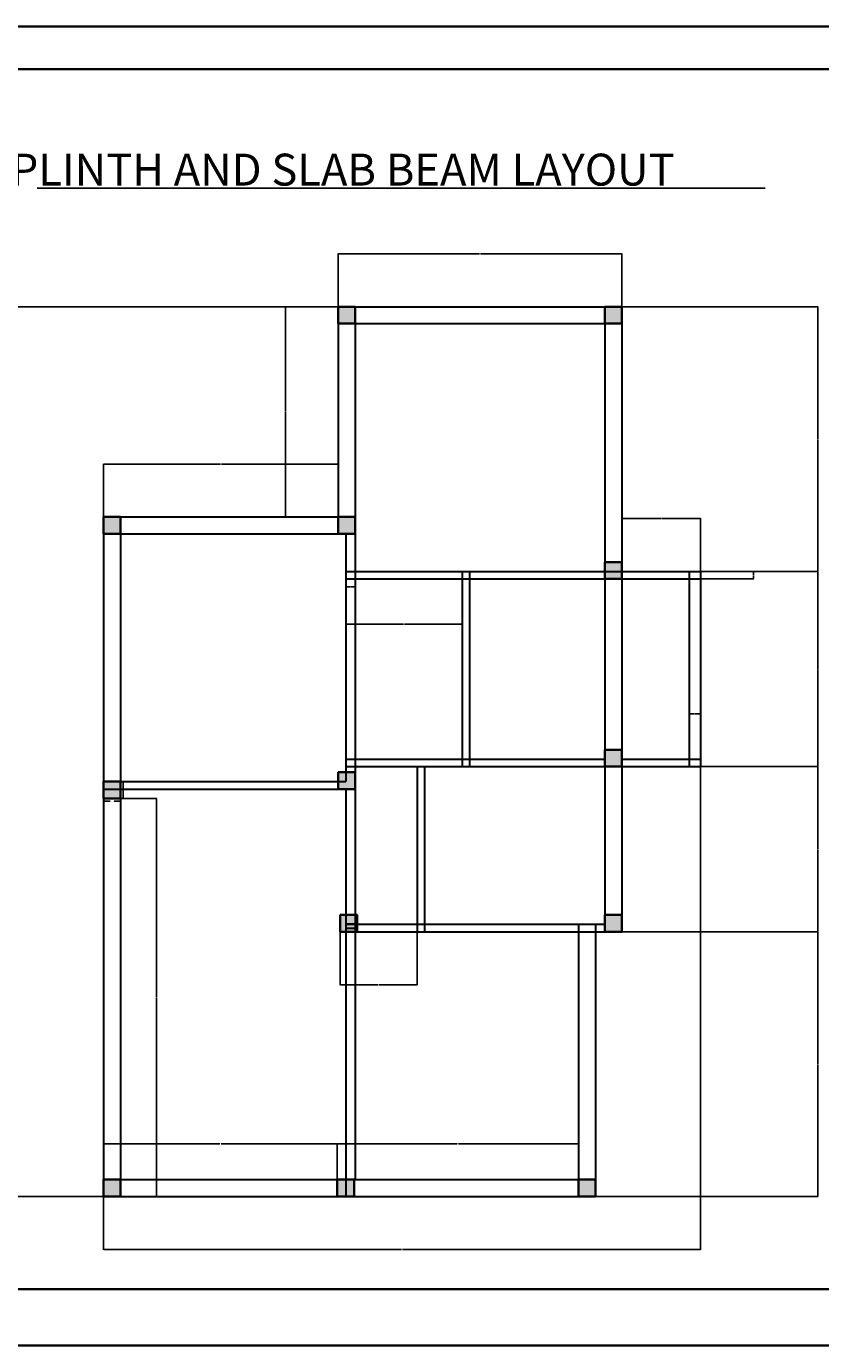
# Model space of a CAD drawing. Units: inches. Extents: x 1762 to 3150, y 1680 to 2382.
# Tile 5 of 6: x 2199 to 2622, y 1680 to 2382. Entities that reach past the tile are written whole.
import ezdxf

# ---------------------------------------------------------------- set-up
doc = ezdxf.new("R2010")
doc.units = ezdxf.units.IN
for name, color, linetype, lineweight in [('A-ANNO-DIMS', 2, 'Continuous', 18), ('A-ANNO-TEXT', 7, 'Continuous', 25), ('A-ANNO-TTLB', 7, 'Continuous', 35), ('S-BEAM', 7, 'Continuous', 30), ('S-COLS', 1, 'Continuous', 35)]:
    doc.layers.add(name, color=color, linetype=linetype, lineweight=lineweight)
doc.styles.get("Standard").update_dxf_attribs({"font": 'arial.ttf'})
doc.dimstyles.get("Standard").update_dxf_attribs({"dimtxt": 0.18, "dimasz": 0.18, "dimexe": 0.18, "dimexo": 0.0625, "dimgap": 0.09, "dimtad": 0, "dimtih": 1, "dimtoh": 1, "dimdec": 4, "dimzin": 0, "dimdsep": 46, "dimtxsty": 'Standard', "dimcen": 0.09, "dimadec": 0, "dimazin": 0, "dimtfac": 1, "dimtdec": 4, "dimtofl": 0, "dimtmove": 0, "dimatfit": 3, "dimfxl": 1, "dimtolj": 1, "dimtzin": 0, "dimarcsym": 0})

# ---------------------------------------------------------------- blocks, each defined once
blk = doc.blocks.new('COL-9X9IN')
h = blk.add_hatch(color=256)
h.dxf.hatch_style = 1
h.paths.add_polyline_path([(0, 0), (9, 0), (9, 9), (0, 9)])
blk.add_lwpolyline([(0, 9), (9, 9), (9, 0), (0, 0)], close=True)
blk = doc.blocks.new('*D30')
at = {"layer": 'A-ANNO-DIMS', "color": 0, "lineweight": -2, "transparency": 16777216}
for p, q in [((2239.94, 1970.93), (2239.94, 1969.46)), ((2240.12, 1969.64), (2243.4, 1969.64)), ((2248.76, 1969.64), (2245.48, 1969.64)), ((2248.94, 1970.93), (2248.94, 1969.46))]:
    blk.add_line(p, q, dxfattribs=at)
at = {"layer": 'A-ANNO-DIMS', "color": 0, "transparency": 16777216}
for points in [[(2240.12, 1969.67), (2240.12, 1969.61), (2239.94, 1969.64)], [(2248.76, 1969.67), (2248.76, 1969.61), (2248.94, 1969.64)]]:
    blk.add_solid(points, dxfattribs=at)
at = {"layer": 'Defpoints', "color": 0, "transparency": 16777216}
for p in [(2239.94, 1970.99), (2248.94, 1970.99), (2248.94, 1969.64)]:
    blk.add_point(p, dxfattribs=at)
at = {"layer": 'A-ANNO-DIMS', "color": 0, "transparency": 16777216, "insert": (2244.44, 1969.64), "char_height": 0.18, "attachment_point": 5}
blk.add_mtext('\\A1;COLUMN 9 TYP.', dxfattribs=at)
blk = doc.blocks.new('*D31')
at = {"layer": 'A-ANNO-DIMS', "color": 0, "lineweight": -2, "transparency": 16777216}
for p, q in [((2249, 1979.99), (2250.47, 1979.99)), ((2250.29, 1979.81), (2250.29, 1975.67)), ((2250.29, 1971.17), (2250.29, 1975.31)), ((2249, 1970.99), (2250.47, 1970.99))]:
    blk.add_line(p, q, dxfattribs=at)
at = {"layer": 'A-ANNO-DIMS', "color": 0, "transparency": 16777216}
for points in [[(2250.26, 1979.81), (2250.32, 1979.81), (2250.29, 1979.99)], [(2250.26, 1971.17), (2250.32, 1971.17), (2250.29, 1970.99)]]:
    blk.add_solid(points, dxfattribs=at)
at = {"layer": 'Defpoints', "color": 0, "transparency": 16777216}
for p in [(2248.94, 1979.99), (2250.29, 1979.99), (2248.94, 1970.99)]:
    blk.add_point(p, dxfattribs=at)
at = {"layer": 'A-ANNO-DIMS', "color": 0, "transparency": 16777216, "insert": (2250.29, 1975.49), "char_height": 0.18, "attachment_point": 5}
blk.add_mtext('\\A1;9 TYP.', dxfattribs=at)
blk = doc.blocks.new('*D64')
at = {"layer": 'A-ANNO-DIMS', "color": 0, "lineweight": -2, "transparency": 16777216}
for p, q in [((2557.94, 1987.93), (2557.94, 1730.66)), ((2239.94, 1758.93), (2239.94, 1730.66)), ((2240.12, 1730.84), (2398.65, 1730.84)), ((2557.76, 1730.84), (2399.23, 1730.84))]:
    blk.add_line(p, q, dxfattribs=at)
at = {"layer": 'A-ANNO-DIMS', "color": 0, "transparency": 16777216}
for points in [[(2240.12, 1730.87), (2240.12, 1730.81), (2239.94, 1730.84)], [(2557.76, 1730.87), (2557.76, 1730.81), (2557.94, 1730.84)]]:
    blk.add_solid(points, dxfattribs=at)
at = {"layer": 'Defpoints', "color": 0, "transparency": 16777216}
for p in [(2557.94, 1987.99), (2239.94, 1758.99), (2557.94, 1730.84)]:
    blk.add_point(p, dxfattribs=at)
at = {"layer": 'A-ANNO-DIMS', "color": 0, "transparency": 16777216, "insert": (2398.94, 1730.84), "char_height": 0.18, "attachment_point": 5}
blk.add_mtext('\\A1;318', dxfattribs=at)
blk = doc.blocks.new('*D65')
at = {"layer": 'A-ANNO-DIMS', "color": 0, "lineweight": -2, "transparency": 16777216}
for p, q in [((2364.876105, 2232.98945), (2176.268936, 2232.98945)), ((2176.448936, 2232.80945), (2176.448936, 1996.16945)), ((2176.448936, 1759.16945), (2176.448936, 1995.80945)), ((2239.876105, 1758.98945), (2176.268936, 1758.98945))]:
    blk.add_line(p, q, dxfattribs=at)
at = {"layer": 'A-ANNO-DIMS', "color": 0, "transparency": 16777216}
for points in [[(2176.418936, 2232.80945), (2176.478936, 2232.80945), (2176.448936, 2232.98945)], [(2176.418936, 1759.16945), (2176.478936, 1759.16945), (2176.448936, 1758.98945)]]:
    blk.add_solid(points, dxfattribs=at)
at = {"layer": 'Defpoints', "color": 0, "transparency": 16777216}
for p in [(2176.448936, 2232.98945), (2364.938605, 2232.98945), (2239.938605, 1758.98945)]:
    blk.add_point(p, dxfattribs=at)
at = {"layer": 'A-ANNO-DIMS', "color": 0, "transparency": 16777216, "insert": (2176.448936, 1995.98945), "char_height": 0.18, "attachment_point": 5}
blk.add_mtext('\\A1;474', dxfattribs=at)
blk = doc.blocks.new('*D66')
at = {"layer": 'A-ANNO-DIMS', "color": 0, "lineweight": -2, "transparency": 16777216}
for p, q in [((2239.94, 2121.05), (2239.94, 2149.32)), ((2240.12, 2149.14), (2302.16, 2149.14)), ((2364.76, 2149.14), (2302.72, 2149.14)), ((2364.94, 2121.05), (2364.94, 2149.32))]:
    blk.add_line(p, q, dxfattribs=at)
at = {"layer": 'A-ANNO-DIMS', "color": 0, "transparency": 16777216}
for points in [[(2240.12, 2149.17), (2240.12, 2149.11), (2239.94, 2149.14)], [(2364.76, 2149.17), (2364.76, 2149.11), (2364.94, 2149.14)]]:
    blk.add_solid(points, dxfattribs=at)
at = {"layer": 'Defpoints', "color": 0, "transparency": 16777216}
for p in [(2364.94, 2149.14), (2239.94, 2120.99), (2364.94, 2120.99)]:
    blk.add_point(p, dxfattribs=at)
at = {"layer": 'A-ANNO-DIMS', "color": 0, "transparency": 16777216, "insert": (2302.44, 2149.14), "char_height": 0.18, "attachment_point": 5}
blk.add_mtext('\\A1;125', dxfattribs=at)
blk = doc.blocks.new('*D67')
at = {"layer": 'A-ANNO-DIMS', "color": 0, "lineweight": -2, "transparency": 16777216}
for p, q in [((2364.94, 2233.05), (2364.94, 2261.32)), ((2365.12, 2261.14), (2440.18, 2261.14)), ((2515.76, 2261.14), (2440.7, 2261.14)), ((2515.94, 2233.05), (2515.94, 2261.32))]:
    blk.add_line(p, q, dxfattribs=at)
at = {"layer": 'A-ANNO-DIMS', "color": 0, "transparency": 16777216}
for points in [[(2365.12, 2261.17), (2365.12, 2261.11), (2364.94, 2261.14)], [(2515.76, 2261.17), (2515.76, 2261.11), (2515.94, 2261.14)]]:
    blk.add_solid(points, dxfattribs=at)
at = {"layer": 'Defpoints', "color": 0, "transparency": 16777216}
for p in [(2515.94, 2261.14), (2364.94, 2232.99), (2515.94, 2232.99)]:
    blk.add_point(p, dxfattribs=at)
at = {"layer": 'A-ANNO-DIMS', "color": 0, "transparency": 16777216, "insert": (2440.44, 2261.14), "char_height": 0.18, "attachment_point": 5}
blk.add_mtext('\\A1;151', dxfattribs=at)
blk = doc.blocks.new('*D68')
at = {"layer": 'A-ANNO-DIMS', "color": 0, "lineweight": -2, "transparency": 16777216}
for p, q in [((2515.94, 2092.05), (2515.94, 2120.32)), ((2516.12, 2120.14), (2536.72, 2120.14)), ((2557.76, 2120.14), (2537.16, 2120.14)), ((2557.94, 2092.05), (2557.94, 2120.32))]:
    blk.add_line(p, q, dxfattribs=at)
at = {"layer": 'A-ANNO-DIMS', "color": 0, "transparency": 16777216}
for points in [[(2516.12, 2120.17), (2516.12, 2120.11), (2515.94, 2120.14)], [(2557.76, 2120.17), (2557.76, 2120.11), (2557.94, 2120.14)]]:
    blk.add_solid(points, dxfattribs=at)
at = {"layer": 'Defpoints', "color": 0, "transparency": 16777216}
for p in [(2557.94, 2120.14), (2515.94, 2091.99), (2557.94, 2091.99)]:
    blk.add_point(p, dxfattribs=at)
at = {"layer": 'A-ANNO-DIMS', "color": 0, "transparency": 16777216, "insert": (2536.94, 2120.14), "char_height": 0.18, "attachment_point": 5}
blk.add_mtext('\\A1;42', dxfattribs=at)
blk = doc.blocks.new('*D69')
at = {"layer": 'A-ANNO-DIMS', "color": 0, "lineweight": -2, "transparency": 16777216}
for p, q in [((2558, 2091.99), (2620.6, 2091.99)), ((2620.42, 2091.81), (2620.42, 2040.17)), ((2620.42, 1988.17), (2620.42, 2039.81)), ((2558, 1987.99), (2620.6, 1987.99))]:
    blk.add_line(p, q, dxfattribs=at)
at = {"layer": 'A-ANNO-DIMS', "color": 0, "transparency": 16777216}
for points in [[(2620.39, 2091.81), (2620.45, 2091.81), (2620.42, 2091.99)], [(2620.39, 1988.17), (2620.45, 1988.17), (2620.42, 1987.99)]]:
    blk.add_solid(points, dxfattribs=at)
at = {"layer": 'Defpoints', "color": 0, "transparency": 16777216}
for p in [(2557.94, 2091.99), (2620.42, 2091.99), (2557.94, 1987.99)]:
    blk.add_point(p, dxfattribs=at)
at = {"layer": 'A-ANNO-DIMS', "color": 0, "transparency": 16777216, "insert": (2620.42, 2039.99), "char_height": 0.18, "attachment_point": 5}
blk.add_mtext('\\A1;104', dxfattribs=at)
blk = doc.blocks.new('*D70')
at = {"layer": 'A-ANNO-DIMS', "color": 0, "lineweight": -2, "transparency": 16777216}
for p, q in [((2516, 1987.99), (2620.6, 1987.99)), ((2620.42, 1987.81), (2620.42, 1944.17)), ((2620.42, 1900.17), (2620.42, 1943.81)), ((2516, 1899.99), (2620.6, 1899.99))]:
    blk.add_line(p, q, dxfattribs=at)
at = {"layer": 'A-ANNO-DIMS', "color": 0, "transparency": 16777216}
for points in [[(2620.39, 1987.81), (2620.45, 1987.81), (2620.42, 1987.99)], [(2620.39, 1900.17), (2620.45, 1900.17), (2620.42, 1899.99)]]:
    blk.add_solid(points, dxfattribs=at)
at = {"layer": 'Defpoints', "color": 0, "transparency": 16777216}
for p in [(2515.94, 1987.99), (2620.42, 1987.99), (2515.94, 1899.99)]:
    blk.add_point(p, dxfattribs=at)
at = {"layer": 'A-ANNO-DIMS', "color": 0, "transparency": 16777216, "insert": (2620.42, 1943.99), "char_height": 0.18, "attachment_point": 5}
blk.add_mtext('\\A1;88', dxfattribs=at)
blk = doc.blocks.new('*D71')
at = {"layer": 'A-ANNO-DIMS', "color": 0, "lineweight": -2, "transparency": 16777216}
for p, q in [((2502, 1899.99), (2620.6, 1899.99)), ((2620.42, 1899.81), (2620.42, 1829.67)), ((2620.42, 1759.17), (2620.42, 1829.31)), ((2502, 1758.99), (2620.6, 1758.99))]:
    blk.add_line(p, q, dxfattribs=at)
at = {"layer": 'A-ANNO-DIMS', "color": 0, "transparency": 16777216}
for points in [[(2620.39, 1899.81), (2620.45, 1899.81), (2620.42, 1899.99)], [(2620.39, 1759.17), (2620.45, 1759.17), (2620.42, 1758.99)]]:
    blk.add_solid(points, dxfattribs=at)
at = {"layer": 'Defpoints', "color": 0, "transparency": 16777216}
for p in [(2501.94, 1899.99), (2620.42, 1899.99), (2501.94, 1758.99)]:
    blk.add_point(p, dxfattribs=at)
at = {"layer": 'A-ANNO-DIMS', "color": 0, "transparency": 16777216, "insert": (2620.42, 1829.49), "char_height": 0.18, "attachment_point": 5}
blk.add_mtext('\\A1;141', dxfattribs=at)
blk = doc.blocks.new('*D72')
at = {"layer": 'A-ANNO-DIMS', "color": 0, "lineweight": -2, "transparency": 16777216}
for p, q in [((2516, 2232.99), (2620.6, 2232.99)), ((2620.42, 2232.81), (2620.42, 2162.67)), ((2620.42, 2092.17), (2620.42, 2162.31)), ((2516, 2091.99), (2620.6, 2091.99))]:
    blk.add_line(p, q, dxfattribs=at)
at = {"layer": 'A-ANNO-DIMS', "color": 0, "transparency": 16777216}
for points in [[(2620.39, 2232.81), (2620.45, 2232.81), (2620.42, 2232.99)], [(2620.39, 2092.17), (2620.45, 2092.17), (2620.42, 2091.99)]]:
    blk.add_solid(points, dxfattribs=at)
at = {"layer": 'Defpoints', "color": 0, "transparency": 16777216}
for p in [(2515.94, 2232.99), (2620.42, 2232.99), (2515.94, 2091.99)]:
    blk.add_point(p, dxfattribs=at)
at = {"layer": 'A-ANNO-DIMS', "color": 0, "transparency": 16777216, "insert": (2620.42, 2162.49), "char_height": 0.18, "attachment_point": 5}
blk.add_mtext('\\A1;141', dxfattribs=at)
blk = doc.blocks.new('*D73')
at = {"layer": 'A-ANNO-DIMS', "color": 0, "lineweight": -2, "transparency": 16777216}
for p, q in [((2364.88, 2232.99), (2336.61, 2232.99)), ((2336.79, 2232.81), (2336.79, 2177.17)), ((2336.79, 2121.17), (2336.79, 2176.81)), ((2364.88, 2120.99), (2336.61, 2120.99))]:
    blk.add_line(p, q, dxfattribs=at)
at = {"layer": 'A-ANNO-DIMS', "color": 0, "transparency": 16777216}
for points in [[(2336.76, 2232.81), (2336.82, 2232.81), (2336.79, 2232.99)], [(2336.76, 2121.17), (2336.82, 2121.17), (2336.79, 2120.99)]]:
    blk.add_solid(points, dxfattribs=at)
at = {"layer": 'Defpoints', "color": 0, "transparency": 16777216}
for p in [(2336.79, 2232.99), (2364.94, 2232.99), (2364.94, 2120.99)]:
    blk.add_point(p, dxfattribs=at)
at = {"layer": 'A-ANNO-DIMS', "color": 0, "transparency": 16777216, "insert": (2336.79, 2176.99), "char_height": 0.18, "attachment_point": 5}
blk.add_mtext('\\A1;112', dxfattribs=at)
blk = doc.blocks.new('*D74')
at = {"layer": 'A-ANNO-DIMS', "color": 0, "lineweight": -2, "transparency": 16777216}
for p, q in [((2240, 1970.99), (2268.27, 1970.99)), ((2268.09, 1970.81), (2268.09, 1865.17)), ((2268.09, 1759.17), (2268.09, 1864.81)), ((2240, 1758.99), (2268.27, 1758.99))]:
    blk.add_line(p, q, dxfattribs=at)
at = {"layer": 'A-ANNO-DIMS', "color": 0, "transparency": 16777216}
for points in [[(2268.06, 1970.81), (2268.12, 1970.81), (2268.09, 1970.99)], [(2268.06, 1759.17), (2268.12, 1759.17), (2268.09, 1758.99)]]:
    blk.add_solid(points, dxfattribs=at)
at = {"layer": 'Defpoints', "color": 0, "transparency": 16777216}
for p in [(2239.94, 1970.99), (2239.94, 1758.99), (2268.09, 1758.99)]:
    blk.add_point(p, dxfattribs=at)
at = {"layer": 'A-ANNO-DIMS', "color": 0, "transparency": 16777216, "insert": (2268.09, 1864.99), "char_height": 0.18, "attachment_point": 5}
blk.add_mtext('\\A1;212', dxfattribs=at)
blk = doc.blocks.new('*D75')
at = {"layer": 'A-ANNO-DIMS', "color": 0, "lineweight": -2, "transparency": 16777216}
for p, q in [((2368.94, 2091.93), (2368.94, 2063.66)), ((2430.94, 2091.93), (2430.94, 2063.66)), ((2369.12, 2063.84), (2399.72, 2063.84)), ((2430.76, 2063.84), (2400.16, 2063.84))]:
    blk.add_line(p, q, dxfattribs=at)
at = {"layer": 'A-ANNO-DIMS', "color": 0, "transparency": 16777216}
for points in [[(2369.12, 2063.87), (2369.12, 2063.81), (2368.94, 2063.84)], [(2430.76, 2063.87), (2430.76, 2063.81), (2430.94, 2063.84)]]:
    blk.add_solid(points, dxfattribs=at)
at = {"layer": 'Defpoints', "color": 0, "transparency": 16777216}
for p in [(2368.94, 2091.99), (2430.94, 2091.99), (2368.94, 2063.84)]:
    blk.add_point(p, dxfattribs=at)
at = {"layer": 'A-ANNO-DIMS', "color": 0, "transparency": 16777216, "insert": (2399.94, 2063.84), "char_height": 0.18, "attachment_point": 5}
blk.add_mtext('\\A1;62', dxfattribs=at)
blk = doc.blocks.new('*D76')
at = {"layer": 'A-ANNO-DIMS', "color": 0, "lineweight": -2, "transparency": 16777216}
for p, q in [((2365.94, 1899.93), (2365.94, 1871.66)), ((2406.94, 1899.93), (2406.94, 1871.66)), ((2366.12, 1871.84), (2386.23, 1871.84)), ((2406.76, 1871.84), (2386.64, 1871.84))]:
    blk.add_line(p, q, dxfattribs=at)
at = {"layer": 'A-ANNO-DIMS', "color": 0, "transparency": 16777216}
for points in [[(2366.12, 1871.87), (2366.12, 1871.81), (2365.94, 1871.84)], [(2406.76, 1871.87), (2406.76, 1871.81), (2406.94, 1871.84)]]:
    blk.add_solid(points, dxfattribs=at)
at = {"layer": 'Defpoints', "color": 0, "transparency": 16777216}
for p in [(2365.94, 1899.99), (2406.94, 1899.99), (2365.94, 1871.84)]:
    blk.add_point(p, dxfattribs=at)
at = {"layer": 'A-ANNO-DIMS', "color": 0, "transparency": 16777216, "insert": (2386.44, 1871.84), "char_height": 0.18, "attachment_point": 5}
blk.add_mtext('\\A1;41', dxfattribs=at)
blk = doc.blocks.new('*D77')
at = {"layer": 'A-ANNO-DIMS', "color": 0, "lineweight": -2, "transparency": 16777216}
for p, q in [((2558.001105, 2091.98945), (2586.268605, 2091.98945)), ((2558.001105, 2087.98945), (2586.268605, 2087.98945)), ((2586.088605, 2091.80945), (2586.088605, 2090.16945)), ((2586.088605, 2088.16945), (2586.088605, 2089.80945))]:
    blk.add_line(p, q, dxfattribs=at)
at = {"layer": 'A-ANNO-DIMS', "color": 0, "transparency": 16777216}
for points in [[(2586.058605, 2091.80945), (2586.118605, 2091.80945), (2586.088605, 2091.98945)], [(2586.058605, 2088.16945), (2586.118605, 2088.16945), (2586.088605, 2087.98945)]]:
    blk.add_solid(points, dxfattribs=at)
at = {"layer": 'Defpoints', "color": 0, "transparency": 16777216}
for p in [(2557.938605, 2091.98945), (2557.938605, 2087.98945), (2586.088605, 2087.98945)]:
    blk.add_point(p, dxfattribs=at)
at = {"layer": 'A-ANNO-DIMS', "color": 0, "transparency": 16777216, "insert": (2586.088605, 2089.98945), "char_height": 0.18, "attachment_point": 5}
blk.add_mtext('\\A1;4', dxfattribs=at)
blk = doc.blocks.new('*D78')
at = {"layer": 'A-ANNO-DIMS', "color": 0, "lineweight": -2, "transparency": 16777216}
for p, q in [((2551.94, 1988.05), (2551.94, 2016.32)), ((2552.12, 2016.14), (2554.79, 2016.14)), ((2557.76, 2016.14), (2555.09, 2016.14)), ((2557.94, 1988.05), (2557.94, 2016.32))]:
    blk.add_line(p, q, dxfattribs=at)
at = {"layer": 'A-ANNO-DIMS', "color": 0, "transparency": 16777216}
for points in [[(2552.12, 2016.17), (2552.12, 2016.11), (2551.94, 2016.14)], [(2557.76, 2016.17), (2557.76, 2016.11), (2557.94, 2016.14)]]:
    blk.add_solid(points, dxfattribs=at)
at = {"layer": 'Defpoints', "color": 0, "transparency": 16777216}
for p in [(2557.94, 2016.14), (2551.94, 1987.99), (2557.94, 1987.99)]:
    blk.add_point(p, dxfattribs=at)
at = {"layer": 'A-ANNO-DIMS', "color": 0, "transparency": 16777216, "insert": (2554.94, 2016.14), "char_height": 0.18, "attachment_point": 5}
blk.add_mtext('\\A1;6', dxfattribs=at)
blk = doc.blocks.new('*D79')
at = {"layer": 'A-ANNO-DIMS', "color": 0, "lineweight": -2, "transparency": 16777216}
for p, q in [((2368.94, 2111.93), (2368.94, 2083.66)), ((2373.94, 2111.93), (2373.94, 2083.66)), ((2369.12, 2083.84), (2371.29, 2083.84)), ((2373.76, 2083.84), (2371.59, 2083.84))]:
    blk.add_line(p, q, dxfattribs=at)
at = {"layer": 'A-ANNO-DIMS', "color": 0, "transparency": 16777216}
for points in [[(2369.12, 2083.87), (2369.12, 2083.81), (2368.94, 2083.84)], [(2373.76, 2083.87), (2373.76, 2083.81), (2373.94, 2083.84)]]:
    blk.add_solid(points, dxfattribs=at)
at = {"layer": 'Defpoints', "color": 0, "transparency": 16777216}
for p in [(2368.94, 2111.99), (2373.94, 2111.99), (2368.94, 2083.84)]:
    blk.add_point(p, dxfattribs=at)
at = {"layer": 'A-ANNO-DIMS', "color": 0, "transparency": 16777216, "insert": (2371.44, 2083.84), "char_height": 0.18, "attachment_point": 5}
blk.add_mtext('\\A1;5', dxfattribs=at)
blk = doc.blocks.new('*D80')
at = {"layer": 'A-ANNO-DIMS', "color": 0, "lineweight": -2, "transparency": 16777216}
for p, q in [((2239.94, 1759.05), (2239.94, 1787.32)), ((2240.12, 1787.14), (2301.8, 1787.14)), ((2364.26, 1787.14), (2302.57, 1787.14)), ((2364.44, 1759.05), (2364.44, 1787.32))]:
    blk.add_line(p, q, dxfattribs=at)
at = {"layer": 'A-ANNO-DIMS', "color": 0, "transparency": 16777216}
for points in [[(2240.12, 1787.17), (2240.12, 1787.11), (2239.94, 1787.14)], [(2364.26, 1787.17), (2364.26, 1787.11), (2364.44, 1787.14)]]:
    blk.add_solid(points, dxfattribs=at)
at = {"layer": 'Defpoints', "color": 0, "transparency": 16777216}
for p in [(2364.44, 1787.14), (2239.94, 1758.99), (2364.44, 1758.99)]:
    blk.add_point(p, dxfattribs=at)
at = {"layer": 'A-ANNO-DIMS', "color": 0, "transparency": 16777216, "insert": (2302.19, 1787.14), "char_height": 0.18, "attachment_point": 5}
blk.add_mtext('\\A1;124.5', dxfattribs=at)
blk = doc.blocks.new('*D81')
at = {"layer": 'A-ANNO-DIMS', "color": 0, "lineweight": -2, "transparency": 16777216}
for p, q in [((2364.44, 1759.05), (2364.44, 1787.32)), ((2364.62, 1787.14), (2428.3, 1787.14)), ((2492.76, 1787.14), (2429.07, 1787.14)), ((2492.94, 1759.05), (2492.94, 1787.32))]:
    blk.add_line(p, q, dxfattribs=at)
at = {"layer": 'A-ANNO-DIMS', "color": 0, "transparency": 16777216}
for points in [[(2364.62, 1787.17), (2364.62, 1787.11), (2364.44, 1787.14)], [(2492.76, 1787.17), (2492.76, 1787.11), (2492.94, 1787.14)]]:
    blk.add_solid(points, dxfattribs=at)
at = {"layer": 'Defpoints', "color": 0, "transparency": 16777216}
for p in [(2492.94, 1787.14), (2364.44, 1758.99), (2492.94, 1758.99)]:
    blk.add_point(p, dxfattribs=at)
at = {"layer": 'A-ANNO-DIMS', "color": 0, "transparency": 16777216, "insert": (2428.69, 1787.14), "char_height": 0.18, "attachment_point": 5}
blk.add_mtext('\\A1;128.5', dxfattribs=at)

msp = doc.modelspace()

# ---------------------------------------------------------------- linework, layer by layer
at = {"layer": 'A-ANNO-TEXT'}
msp.add_line((2204.5989, 2296.1738), (2592.2662, 2296.1738), dxfattribs=at)
at = {"layer": 'A-ANNO-TTLB'}
for points in [[(1762.4998, 2382.3025), (3150.3176, 2382.3025), (3150.3176, 1679.5742), (1762.4998, 1679.5742)], [(1799.0337, 2359.5805), (3111.4319, 2359.5805), (3111.4319, 1709.6712), (1799.0337, 1709.6712)]]:
    msp.add_lwpolyline(points, close=True, dxfattribs=at)
at = {"layer": 'S-BEAM'}
for p, q in [((2364.9386, 2232.9895), (2515.9386, 2232.9895)), ((2364.9386, 2232.9895), (2364.9386, 2223.9895)), ((2364.9386, 2232.9895), (2364.9386, 2120.9895)), ((2373.9386, 2232.9895), (2373.9386, 2087.9895)), ((2506.9386, 2232.9895), (2506.9386, 2091.9895)), ((2515.9386, 2232.9895), (2515.9386, 2091.9895)), ((2364.9386, 2223.9895), (2515.9386, 2223.9895)), ((2364.9386, 2223.9895), (2364.9386, 2120.9895)), ((2239.9386, 2120.9895), (2364.9386, 2120.9895)), ((2239.9386, 2120.9895), (2239.9386, 1758.9895)), ((2239.9386, 2111.9895), (2368.9386, 2111.9895)), ((2248.9386, 2111.9895), (2248.9386, 1979.9895)), ((2368.9386, 2111.9895), (2368.9386, 2039.9895)), ((2368.9386, 2111.9895), (2368.9386, 1984.9895)), ((2368.9386, 2091.9895), (2515.9386, 2091.9895)), ((2368.9386, 2087.9895), (2515.9386, 2087.9895)), ((2373.9386, 2091.9895), (2375.9386, 2091.9895)), ((2373.9386, 2087.9895), (2375.9386, 2087.9895)), ((2373.9386, 2087.9895), (2373.9386, 1767.9895)), ((2430.9386, 2091.9895), (2557.9386, 2091.9895)), ((2430.9386, 2091.9895), (2430.9386, 1987.9895)), ((2434.9386, 2091.9895), (2434.9386, 1987.9895)), ((2506.9386, 2087.9895), (2506.9386, 1991.9895)), ((2515.9386, 2087.9895), (2557.9386, 2087.9895)), ((2515.9386, 2087.9895), (2515.9386, 1987.9895)), ((2551.9386, 2091.9895), (2551.9386, 1987.9895)), ((2557.9386, 2091.9895), (2557.9386, 1987.9895)), ((2368.9386, 1991.9895), (2506.9386, 1991.9895)), ((2368.9386, 1991.9895), (2368.9386, 1979.9895)), ((2368.9386, 1991.9895), (2368.9386, 1979.9895)), ((2515.9386, 1991.9895), (2557.9386, 1991.9895)), ((2368.9386, 1987.9895), (2506.9386, 1987.9895)), ((2406.9386, 1987.9895), (2406.9386, 1945.9895)), ((2410.9386, 1987.9895), (2410.9386, 1945.9895)), ((2506.9386, 1987.9895), (2557.9386, 1987.9895)), ((2506.9386, 1987.9895), (2506.9386, 1903.9895)), ((2515.9386, 1987.9895), (2515.9386, 1899.9895)), ((2239.9386, 1979.9895), (2368.9386, 1979.9895)), ((2239.9386, 1975.9895), (2373.9386, 1975.9895)), ((2248.9386, 1975.9895), (2248.9386, 1758.9895)), ((2368.9386, 1975.9895), (2368.9386, 1758.9895)), ((2406.9386, 1945.9895), (2406.9386, 1899.9895)), ((2410.9386, 1945.9895), (2410.9386, 1899.9895)), ((2365.9386, 1899.9895), (2501.9386, 1899.9895)), ((2368.9386, 1903.9895), (2373.9386, 1903.9895)), ((2368.9386, 1903.9895), (2506.9386, 1903.9895)), ((2374.9386, 1903.9895), (2368.9386, 1903.9895)), ((2368.9386, 1901.9895), (2373.9386, 1901.9895)), ((2372.9386, 1899.9895), (2374.9386, 1899.9895)), ((2374.9386, 1903.9895), (2374.9386, 1899.9895)), ((2492.9386, 1903.9895), (2492.9386, 1758.9895)), ((2501.9386, 1903.9895), (2501.9386, 1758.9895)), ((2501.9386, 1899.9895), (2515.9386, 1899.9895)), ((2239.9386, 1767.9895), (2492.9386, 1767.9895)), ((2364.4386, 1767.9895), (2366.4386, 1767.9895)), ((2372.9386, 1767.9895), (2492.9386, 1767.9895)), ((2239.9386, 1758.9895), (2492.9386, 1758.9895)), ((2366.9386, 1758.9895), (2501.9386, 1758.9895))]:
    msp.add_line(p, q, dxfattribs=at)

# ---------------------------------------------------------------- block references
at = {"layer": 'S-COLS'}
for p in [(2364.939, 2223.989), (2506.939, 2223.989), (2239.939, 2111.989), (2364.939, 2111.989), (2506.939, 2087.989), (2506.939, 1987.989), (2364.939, 1975.989), (2239.939, 1970.989), (2365.939, 1899.989), (2506.939, 1899.989), (2239.939, 1758.989), (2364.439, 1758.989), (2492.939, 1758.989)]:
    msp.add_blockref('COL-9X9IN', p, dxfattribs=at)

# ---------------------------------------------------------------- texts
at = {"layer": 'A-ANNO-TEXT'}
msp.add_text('            PLINTH AND SLAB BEAM LAYOUT', height=17, dxfattribs=at).set_placement((2128.1301, 2297.5007))

# ---------------------------------------------------------------- dimensions: what is measured, and where the dimension line sits
at = {"layer": 'A-ANNO-DIMS'}
for base, p1, p2, override, picture, middle in [((2515.9386, 2261.1395), (2364.9386, 2232.9895), (2515.9386, 2232.9895), {"dimdec": 0, "dimlfac": 1, "dimrnd": 0, "dimzin": 0, "dimdsep": 46, "dimlunit": 2}, '*D67', (2440.4386, 2261.1395)), ((2364.9386, 2149.1395), (2239.9386, 2120.9895), (2364.9386, 2120.9895), {"dimdec": 0, "dimlfac": 1, "dimrnd": 0, "dimzin": 0, "dimdsep": 46, "dimlunit": 2}, '*D66', (2302.4386, 2149.1395)), ((2557.9386, 2120.1395), (2515.9386, 2091.9895), (2557.9386, 2091.9895), {"dimdec": 0, "dimlfac": 1, "dimrnd": 0, "dimzin": 0, "dimdsep": 46, "dimlunit": 2}, '*D68', (2536.9386, 2120.1395)), ((2557.9386, 2016.1394), (2551.9386, 1987.9895), (2557.9386, 1987.9895), {"dimdec": 0, "dimlfac": 1, "dimrnd": 0, "dimzin": 0, "dimdsep": 46, "dimlunit": 2}, '*D78', (2554.9386, 2016.1394)), ((2557.9386, 1730.8394), (2239.9386, 1758.9895), (2557.9386, 1987.9895), {"dimdec": 0, "dimlfac": 1, "dimrnd": 0, "dimzin": 0, "dimdsep": 46, "dimlunit": 2}, '*D64', (2398.9386, 1730.8394)), ((2492.9386, 1787.1394), (2364.4386, 1758.9895), (2492.9386, 1758.9895), {"dimdec": 1, "dimlfac": 1, "dimrnd": 0, "dimzin": 0, "dimdsep": 46, "dimlunit": 2}, '*D81', (2428.6886, 1787.1394))]:
    dim = msp.add_linear_dim(base=base, p1=p1, p2=p2, dimstyle='Standard', override=override, dxfattribs=at)
    dim.commit()
    dim.dimension.update_dxf_attribs({"geometry": picture, "text_midpoint": middle})
for base, p1, p2, angle, override, picture, middle in [((2176.4489, 2232.9895), (2239.9386, 1758.9895), (2364.9386, 2232.9895), 90, {"dimdec": 0, "dimlfac": 1, "dimrnd": 0, "dimzin": 0, "dimdsep": 46, "dimlunit": 2}, '*D65', (2176.4489, 1995.9894)), ((2336.7886, 2232.9895), (2364.9386, 2120.9895), (2364.9386, 2232.9895), 90, {"dimdec": 0, "dimlfac": 1, "dimrnd": 0, "dimzin": 0, "dimdsep": 46, "dimlunit": 2}, '*D73', (2336.7886, 2176.9895)), ((2620.4162, 2232.9895), (2515.9386, 2091.9895), (2515.9386, 2232.9895), 90, {"dimdec": 0, "dimlfac": 1, "dimrnd": 0, "dimzin": 0, "dimdsep": 46, "dimlunit": 2}, '*D72', (2620.4162, 2162.4895)), ((2368.9386, 2083.8394), (2373.9386, 2111.9895), (2368.9386, 2111.9895), 180, {"dimdec": 0, "dimlfac": 1, "dimrnd": 0, "dimzin": 0, "dimdsep": 46, "dimlunit": 2}, '*D79', (2371.4386, 2083.8394)), ((2368.9386, 2063.8395), (2430.9386, 2091.9895), (2368.9386, 2091.9895), 180, {"dimdec": 0, "dimlfac": 1, "dimrnd": 0, "dimzin": 0, "dimdsep": 46, "dimlunit": 2}, '*D75', (2399.9386, 2063.8394)), ((2620.4162, 2091.9895), (2557.9386, 1987.9895), (2557.9386, 2091.9895), 90, {"dimdec": 0, "dimlfac": 1, "dimrnd": 0, "dimzin": 0, "dimdsep": 46, "dimlunit": 2}, '*D69', (2620.4162, 2039.9895)), ((2586.0886, 2087.9895), (2557.9386, 2091.9895), (2557.9386, 2087.9895), 270, {"dimdec": 0, "dimlfac": 1, "dimrnd": 0, "dimzin": 0, "dimdsep": 46, "dimlunit": 2}, '*D77', (2586.0886, 2089.9895)), ((2620.4162, 1987.9895), (2515.9386, 1899.9895), (2515.9386, 1987.9895), 90, {"dimdec": 0, "dimlfac": 1, "dimrnd": 0, "dimzin": 0, "dimdsep": 46, "dimlunit": 2}, '*D70', (2620.4162, 1943.9895)), ((2268.0886, 1758.9895), (2239.9386, 1970.9895), (2239.9386, 1758.9895), 270, {"dimdec": 0, "dimlfac": 1, "dimrnd": 0, "dimzin": 0, "dimdsep": 46, "dimlunit": 2}, '*D74', (2268.0886, 1864.9895)), ((2365.9386, 1871.8394), (2406.9386, 1899.9895), (2365.9386, 1899.9895), 180, {"dimdec": 0, "dimlfac": 1, "dimrnd": 0, "dimzin": 0, "dimdsep": 46, "dimlunit": 2}, '*D76', (2386.4386, 1871.8394)), ((2620.4162, 1899.9895), (2501.9386, 1758.9895), (2501.9386, 1899.9895), 90, {"dimdec": 0, "dimlfac": 1, "dimrnd": 0, "dimzin": 0, "dimdsep": 46, "dimlunit": 2}, '*D71', (2620.4162, 1829.4895)), ((2364.4386, 1787.1394), (2239.9386, 1758.9895), (2364.4386, 1758.9895), 0, {"dimdec": 1, "dimlfac": 1, "dimrnd": 0, "dimzin": 0, "dimdsep": 46, "dimlunit": 2}, '*D80', (2302.1886, 1787.1394))]:
    dim = msp.add_linear_dim(base=base, p1=p1, p2=p2, angle=angle, dimstyle='Standard', override=override, dxfattribs=at)
    dim.commit()
    dim.dimension.update_dxf_attribs({"geometry": picture, "text_midpoint": middle})
dim = msp.add_linear_dim(base=(2250.2886, 1979.9895), p1=(2248.9386, 1970.9895), p2=(2248.9386, 1979.9895), angle=90, text='<> TYP.', dimstyle='Standard', override={"dimdec": 0, "dimlfac": 1, "dimrnd": 0, "dimzin": 0, "dimdsep": 46, "dimlunit": 2}, dxfattribs=at)
dim.commit()
dim.dimension.update_dxf_attribs({"geometry": '*D31', "text_midpoint": (2250.2886, 1975.4895)})
dim = msp.add_linear_dim(base=(2248.9386, 1969.6395), p1=(2239.9386, 1970.9895), p2=(2248.9386, 1970.9895), text='COLUMN <> TYP.', dimstyle='Standard', override={"dimdec": 0, "dimlfac": 1, "dimrnd": 0, "dimzin": 0, "dimdsep": 46, "dimlunit": 2}, dxfattribs=at)
dim.commit()
dim.dimension.update_dxf_attribs({"geometry": '*D30', "text_midpoint": (2244.4386, 1969.6395)})

doc.saveas('drawing.dxf')
